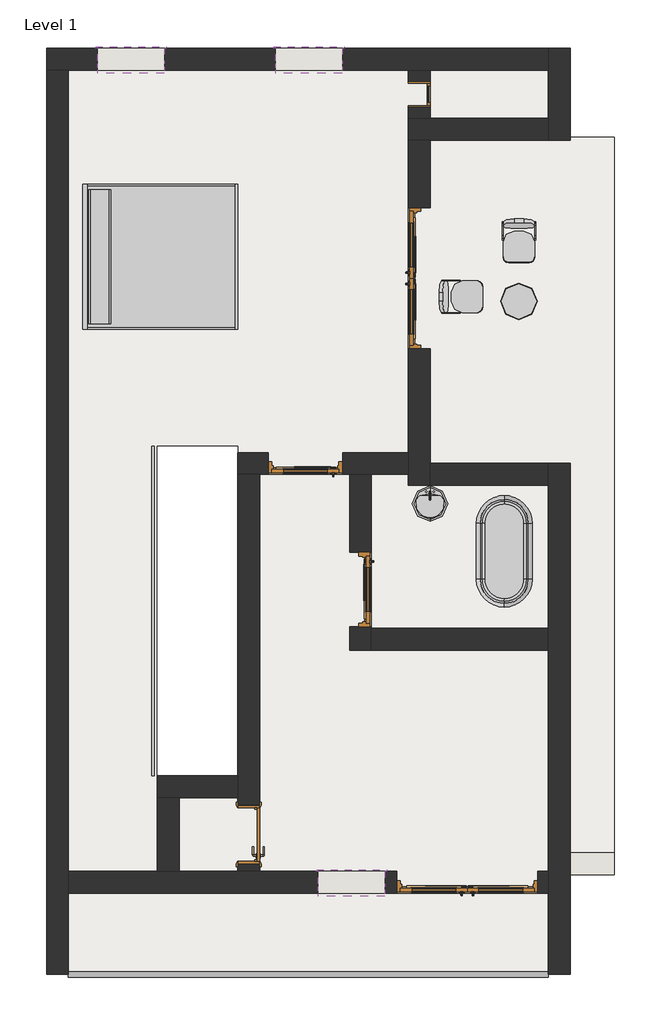
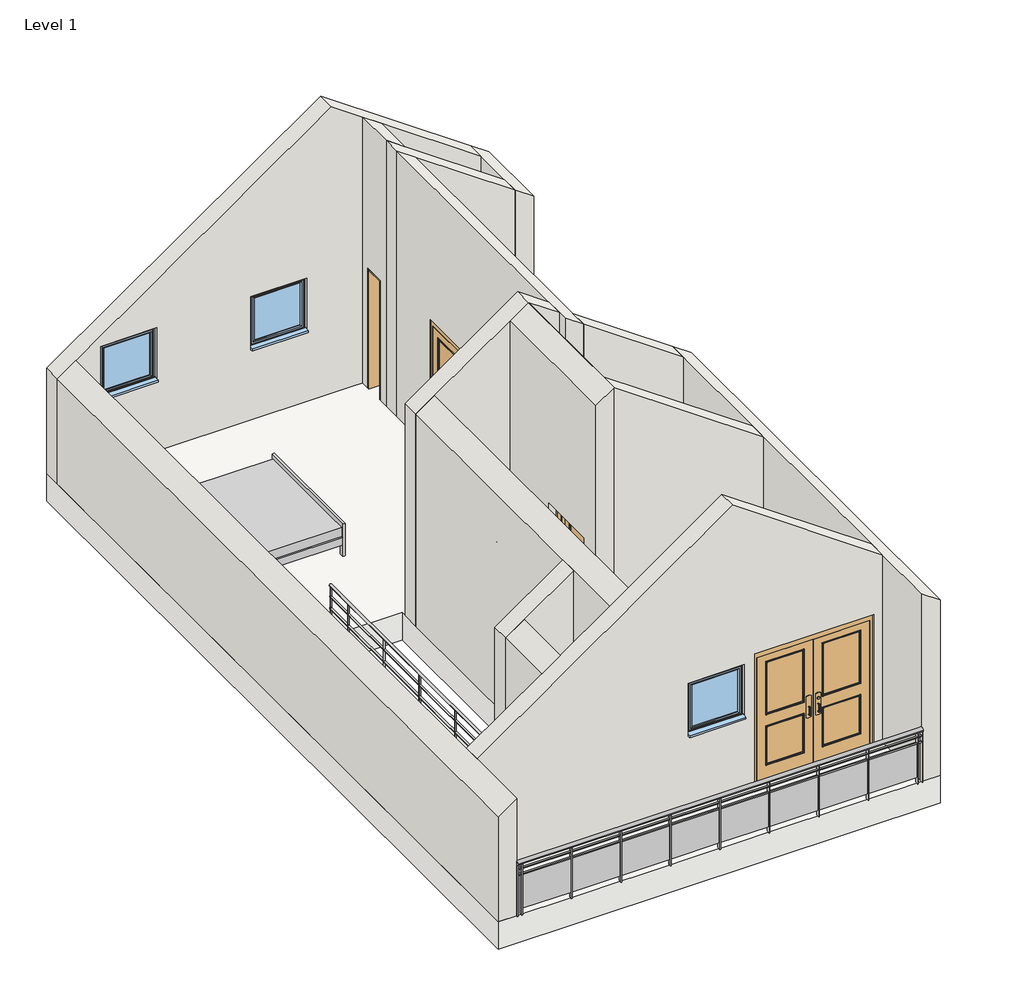
# One storey: 16 walls, 6 doors, 4 furniture elements, 3 windows, 2 flow terminals, 2 railings, 1 slab.
# Revit data of these elements (continued)
# Element 34 (IfcWindow, "Windows_Sgl_Plain : 910x910mm")
#   Mark = "8"
#   Phase Created = New Construction
#   Materials on its faces: "Window Frame", "Glass"
# Materials
#   "Cherry": class "Wood", colour RGB 226 177 128, transparency 0, Description = "Prunus Serotina", Cost = 0
#   "Glass": class "Glass", colour RGB 0 128 192, transparency 0.9, Description = "Soda Lime Glass", Cost = 0
#   "Metal - Stainless Steel": class "Metal", colour RGB 247 247 247, transparency 0
#   "Metal - Painted - Grey": class "Paint", colour RGB 104 104 104, transparency 0
#   "Door - Handle": colour RGB 0 0 0, transparency 0, Keynote = "P21", Cost = 0
#   "Door - Frame/Mullion (1)": class "Wood", colour RGB 212 179 113, transparency 0, Keynote = "L20", Cost = 0
#   "Door - Panel": class "Wood", colour RGB 210 159 95, transparency 0, Keynote = "L20", Cost = 0
#   "Door - Architrave": class "Wood", colour RGB 154 90 5, transparency 0, Keynote = "P20", Cost = 0
#   "Porcelain, Linen": class "Ceramic", colour RGB 249 239 230, transparency 0, Description = "Porcelain, linen", Cost = 0
#   "Steel, Polished": class "Metal", colour RGB 57 57 57, transparency 0, Description = "Polished steel", Cost = 0
#   "Porcelain, Ivory": class "Ceramic", colour RGB 247 247 239, transparency 0, Description = "Porcelain, ivory", Cost = 0
#   "Birch": class "Wood", colour RGB 224 178 126, transparency 0, Description = "Betula Alleghaniensis", Cost = 0
#   "Linen, White": class "Textile", colour RGB 247 247 239, transparency 0, Description = "Linen, white", Cost = 0
#   "Linen, Beige": class "Textile", colour RGB 249 239 230, transparency 0, Description = "Linen, beige", Cost = 0
#   "Steel, Paint Finish, Dark Gray, Matte": class "Metal", colour RGB 98 98 98, transparency 0, Description = "Steel, paint finish, dark gray, matte", Cost = 0
#   "Wood - Birch": colour RGB 230 196 162, transparency 0
#   "Laminate - Ivory,Matte": colour RGB 247 247 239, transparency 0
#   "Concrete, Sand/Cement Screed": class "Concrete", colour RGB 127 127 127, transparency 0, Description = "Concrete slab topping", Cost = 0
#   "Vapor Retarder": class "Generic", colour RGB 120 120 120, transparency 0, Description = "Polyethylene film membrane", Cost = 0
#   "Rigid insulation": class "Generic", colour RGB 127 127 127, transparency 0, Description = "Rigid foam insulation board", Cost = 0
#   "Air": class "Gas", colour RGB 255 255 255, transparency 0, Description = "Air", Cost = 0
#   "Damp-proofing": class "Generic", colour RGB 127 127 127, transparency 0, Description = "Damp-proofing", Cost = 0
#   "Concrete Masonry, Floor Block": class "Concrete", colour RGB 181 181 181, transparency 0, Description = "physical material", Cost = 0
#   "Concrete, Precast": class "Concrete", colour RGB 192 192 192, transparency 0, Description = "Precast concrete", Cost = 0
#   "Concrete, Cast In Situ": class "Concrete", colour RGB 192 192 192, transparency 0, Description = "physical material", Cost = 0
#   "Window Frame": colour RGB 249 249 249, transparency 0, Keynote = "L10", Cost = 0
#   "Door - Frame/Mullion": class "Wood", colour RGB 212 179 113, transparency 0, Keynote = "L20", Cost = 0
#   "Metal - Stainless Steel,Polished": class "Metal", colour RGB 236 239 239, transparency 0, Cost = 0
